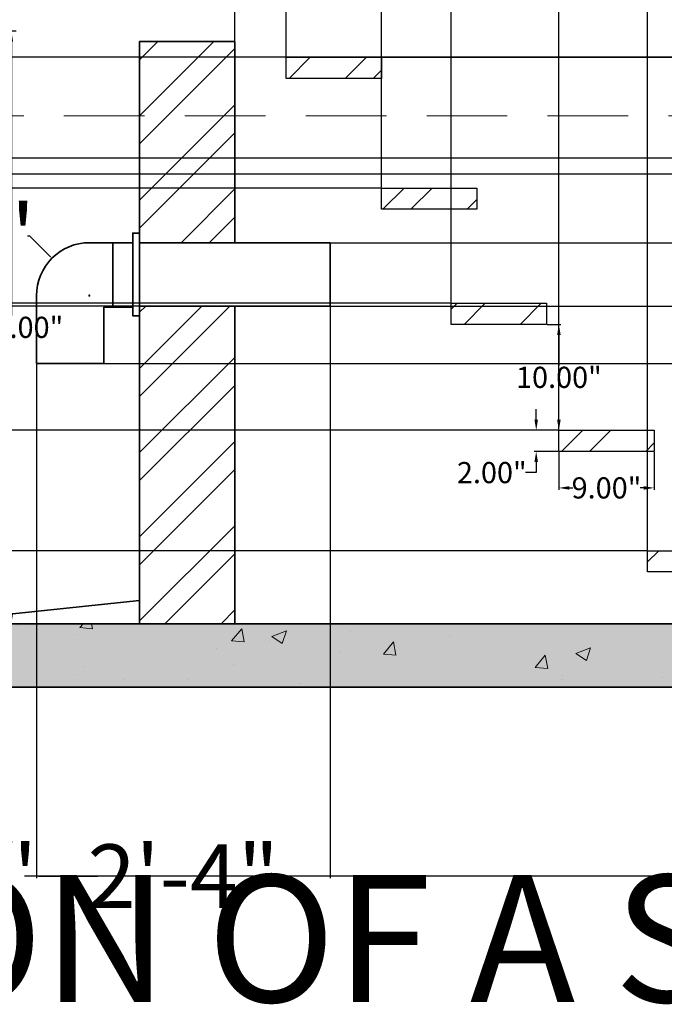
# Model space of a CAD drawing. Units: inches. Extents: x -34 to 285, y -151 to 155.
# Tile 6 of 10: x 129 to 189, y -151 to -58. Entities that reach past the tile are written whole.
import ezdxf

# ---------------------------------------------------------------- set-up
doc = ezdxf.new("R2010")
doc.units = ezdxf.units.IN
doc.header["$MEASUREMENT"] = 0
doc.linetypes.add('DASHED', pattern=[19.05, 12.7, -6.35])
for name, color, linetype, lineweight in [('A-ANNO-DIMS', 2, 'Continuous', 18), ('A-ANNO-TEXT', 7, 'Continuous', 25), ('A-DETL', 7, 'Continuous', 35), ('A-DETL-HIDN', 8, 'DASHED', 18), ('A-DETL-PATT', 8, 'Continuous', 18), ('A-FLOR-STRS', 3, 'Continuous', 25), ('P-SANR-PIPE', 4, 'Continuous', 35)]:
    doc.layers.add(name, color=color, linetype=linetype, lineweight=lineweight)
doc.styles.get("Standard").update_dxf_attribs({"font": 'arial.ttf'})
doc.dimstyles.get("Standard").update_dxf_attribs({"dimtxt": 6, "dimasz": 0.18, "dimexe": 0.18, "dimexo": 0.0625, "dimgap": 0.09, "dimtad": 0, "dimtih": 1, "dimtoh": 1, "dimzin": 0, "dimdsep": 46, "dimlunit": 3, "dimtxsty": 'Standard', "dimcen": 0.09, "dimadec": 0, "dimazin": 0, "dimtfac": 1, "dimtofl": 0, "dimtmove": 0, "dimatfit": 3, "dimfxl": 1, "dimtolj": 1, "dimtzin": 0, "dimarcsym": 0})

# ---------------------------------------------------------------- blocks, each defined once
blk = doc.blocks.new('*D29')
at = {"layer": 'A-ANNO-DIMS', "color": 0, "lineweight": -2, "transparency": 16777216}
for p, q in [((128.176, -58.969), (127.544, -58.969)), ((127.724, -59.969), (127.724, -85.858)), ((127.724, -113.969), (127.724, -88.08)), ((128.176, -114.969), (127.544, -114.969))]:
    blk.add_line(p, q, dxfattribs=at)
at = {"layer": 'A-ANNO-DIMS', "color": 0, "transparency": 16777216}
for points in [[(127.557, -59.969), (127.891, -59.969), (127.724, -58.969)], [(127.557, -113.969), (127.891, -113.969), (127.724, -114.969)]]:
    blk.add_solid(points, dxfattribs=at)
at = {"layer": 'Defpoints', "color": 0, "transparency": 16777216}
for p in [(128.239, -58.969), (127.724, -114.969), (128.239, -114.969)]:
    blk.add_point(p, dxfattribs=at)
at = {"layer": 'A-ANNO-DIMS', "color": 0, "transparency": 16777216, "insert": (127.724, -86.969), "char_height": 2, "attachment_point": 5}
blk.add_mtext('\\A1;4\'-8.00"', dxfattribs=at)
blk = doc.blocks.new('*D32')
at = {"layer": 'A-ANNO-DIMS', "color": 0, "lineweight": -2, "transparency": 16777216}
for p, q in [((178.365, -86.693), (179.662, -86.693)), ((179.482, -87.693), (179.482, -90.582)), ((179.482, -95.693), (179.482, -92.804)), ((179.544, -96.693), (179.662, -96.693))]:
    blk.add_line(p, q, dxfattribs=at)
at = {"layer": 'A-ANNO-DIMS', "color": 0, "transparency": 16777216}
for points in [[(179.315, -87.693), (179.648, -87.693), (179.482, -86.693)], [(179.315, -95.693), (179.648, -95.693), (179.482, -96.693)]]:
    blk.add_solid(points, dxfattribs=at)
at = {"layer": 'Defpoints', "color": 0, "transparency": 16777216}
for p in [(178.303, -86.693), (179.482, -96.693), (179.482, -96.693)]:
    blk.add_point(p, dxfattribs=at)
at = {"layer": 'A-ANNO-DIMS', "color": 0, "transparency": 16777216, "insert": (179.482, -91.693), "char_height": 2, "attachment_point": 5}
blk.add_mtext('\\A1;10.00"', dxfattribs=at)
blk = doc.blocks.new('*D33')
at = {"layer": 'A-ANNO-DIMS', "color": 0, "lineweight": -2, "transparency": 16777216}
for p, q in [((179.482, -98.755), (179.482, -102.319)), ((188.482, -98.755), (188.482, -102.319)), ((180.482, -102.139), (180.8, -102.139)), ((187.482, -102.139), (187.163, -102.139))]:
    blk.add_line(p, q, dxfattribs=at)
at = {"layer": 'A-ANNO-DIMS', "color": 0, "transparency": 16777216}
for points in [[(180.482, -101.973), (180.482, -102.306), (179.482, -102.139)], [(187.482, -101.973), (187.482, -102.306), (188.482, -102.139)]]:
    blk.add_solid(points, dxfattribs=at)
at = {"layer": 'Defpoints', "color": 0, "transparency": 16777216}
for p in [(179.482, -98.693), (188.482, -98.693), (188.482, -102.139)]:
    blk.add_point(p, dxfattribs=at)
at = {"layer": 'A-ANNO-DIMS', "color": 0, "transparency": 16777216, "insert": (183.982, -102.139), "char_height": 2, "attachment_point": 5}
blk.add_mtext('\\A1;9.00"', dxfattribs=at)
blk = doc.blocks.new('*D34')
at = {"layer": 'A-ANNO-DIMS', "color": 0, "lineweight": -2, "transparency": 16777216}
for p, q in [((177.338, -95.693), (177.338, -94.693)), ((179.419, -96.693), (177.158, -96.693)), ((179.419, -98.693), (177.158, -98.693)), ((177.338, -99.693), (177.338, -100.693)), ((177.338, -100.693), (176.338, -100.693))]:
    blk.add_line(p, q, dxfattribs=at)
at = {"layer": 'A-ANNO-DIMS', "color": 0, "transparency": 16777216}
for points in [[(177.171, -95.693), (177.504, -95.693), (177.338, -96.693)], [(177.171, -99.693), (177.504, -99.693), (177.338, -98.693)]]:
    blk.add_solid(points, dxfattribs=at)
at = {"layer": 'Defpoints', "color": 0, "transparency": 16777216}
for p in [(179.482, -96.693), (177.338, -98.693), (179.482, -98.693)]:
    blk.add_point(p, dxfattribs=at)
at = {"layer": 'A-ANNO-DIMS', "color": 0, "transparency": 16777216, "insert": (173.139, -100.693), "char_height": 2, "attachment_point": 5}
blk.add_mtext('\\A1;2.00"', dxfattribs=at)
blk = doc.blocks.new('*D48')
at = {"layer": 'A-ANNO-DIMS', "color": 0, "lineweight": -2, "transparency": 16777216}
for p, q in [((22.846, -121.031), (22.846, -138.999)), ((214.846, -121.031), (214.846, -138.999)), ((23.026, -138.819), (108.733, -138.819)), ((214.666, -138.819), (128.959, -138.819))]:
    blk.add_line(p, q, dxfattribs=at)
at = {"layer": 'A-ANNO-DIMS', "color": 0, "transparency": 16777216}
for points in [[(23.026, -138.789), (23.026, -138.849), (22.846, -138.819)], [(214.666, -138.789), (214.666, -138.849), (214.846, -138.819)]]:
    blk.add_solid(points, dxfattribs=at)
at = {"layer": 'Defpoints', "color": 0, "transparency": 16777216}
for p in [(22.846, -120.969), (214.846, -120.969), (214.846, -138.819)]:
    blk.add_point(p, dxfattribs=at)
at = {"layer": 'A-ANNO-DIMS', "color": 0, "transparency": 16777216, "insert": (118.846, -138.819), "char_height": 6, "attachment_point": 5}
blk.add_mtext('\\A1;16\'-0"', dxfattribs=at)
blk = doc.blocks.new('*D59')
at = {"layer": 'A-ANNO-DIMS', "color": 0, "lineweight": -2, "transparency": 16777216}
for p, q in [((83.148, -48.969), (241.637, -48.969)), ((241.457, -49.149), (241.457, -52)), ((241.457, -61.235), (241.457, -58.384)), ((89.009, -61.415), (241.637, -61.415))]:
    blk.add_line(p, q, dxfattribs=at)
at = {"layer": 'A-ANNO-DIMS', "color": 0, "transparency": 16777216}
for points in [[(241.427, -49.149), (241.487, -49.149), (241.457, -48.969)], [(241.427, -61.235), (241.487, -61.235), (241.457, -61.415)]]:
    blk.add_solid(points, dxfattribs=at)
at = {"layer": 'Defpoints', "color": 0, "transparency": 16777216}
for p in [(83.086, -48.969), (88.947, -61.415), (241.457, -61.415)]:
    blk.add_point(p, dxfattribs=at)
at = {"layer": 'A-ANNO-DIMS', "color": 0, "transparency": 16777216, "insert": (241.457, -55.192), "char_height": 6, "attachment_point": 5}
blk.add_mtext('\\A1;1\'-0 1/2"', dxfattribs=at)
blk = doc.blocks.new('*D61')
at = {"layer": 'A-ANNO-DIMS', "color": 0, "lineweight": -2, "transparency": 16777216}
for p, q in [((148.846, -59.906), (148.846, -18.978)), ((149.026, -19.158), (153.535, -19.158)), ((153.715, -61.389), (153.715, -18.978)), ((153.715, -19.158), (153.895, -19.158))]:
    blk.add_line(p, q, dxfattribs=at)
at = {"layer": 'A-ANNO-DIMS', "color": 0, "transparency": 16777216}
for points in [[(149.026, -19.128), (149.026, -19.188), (148.846, -19.158)], [(153.535, -19.128), (153.535, -19.188), (153.715, -19.158)]]:
    blk.add_solid(points, dxfattribs=at)
at = {"layer": 'Defpoints', "color": 0, "transparency": 16777216}
for p in [(153.715, -19.158), (148.846, -59.969), (153.715, -61.451)]:
    blk.add_point(p, dxfattribs=at)
at = {"layer": 'A-ANNO-DIMS', "color": 0, "transparency": 16777216, "insert": (161.96, -19.158), "char_height": 6, "attachment_point": 5}
blk.add_mtext('\\A1;0\'-5"', dxfattribs=at)
blk = doc.blocks.new('*D62')
at = {"layer": 'A-ANNO-DIMS', "color": 0, "lineweight": -2, "transparency": 16777216}
for p, q in [((155.218, -48.969), (241.637, -48.969)), ((241.457, -49.149), (241.457, -52.018)), ((241.457, -61.271), (241.457, -58.402)), ((153.777, -61.451), (241.637, -61.451))]:
    blk.add_line(p, q, dxfattribs=at)
at = {"layer": 'A-ANNO-DIMS', "color": 0, "transparency": 16777216}
for points in [[(241.427, -49.149), (241.487, -49.149), (241.457, -48.969)], [(241.427, -61.271), (241.487, -61.271), (241.457, -61.451)]]:
    blk.add_solid(points, dxfattribs=at)
at = {"layer": 'Defpoints', "color": 0, "transparency": 16777216}
for p in [(155.156, -48.969), (153.715, -61.451), (241.457, -61.451)]:
    blk.add_point(p, dxfattribs=at)
at = {"layer": 'A-ANNO-DIMS', "color": 0, "transparency": 16777216, "insert": (241.457, -55.21), "char_height": 6, "attachment_point": 5}
blk.add_mtext('\\A1;1\'-0 1/2"', dxfattribs=at)
blk = doc.blocks.new('*D63')
at = {"layer": 'A-ANNO-DIMS', "color": 0, "lineweight": -2, "transparency": 16777216}
for p, q in [((157.846, -79.031), (157.846, -138.999)), ((130.096, -90.432), (130.096, -138.999)), ((130.276, -138.819), (135.855, -138.819)), ((157.666, -138.819), (152.087, -138.819))]:
    blk.add_line(p, q, dxfattribs=at)
at = {"layer": 'A-ANNO-DIMS', "color": 0, "transparency": 16777216}
for points in [[(130.276, -138.789), (130.276, -138.849), (130.096, -138.819)], [(157.666, -138.789), (157.666, -138.849), (157.846, -138.819)]]:
    blk.add_solid(points, dxfattribs=at)
at = {"layer": 'Defpoints', "color": 0, "transparency": 16777216}
for p in [(157.846, -78.969), (130.096, -90.369), (157.846, -138.819)]:
    blk.add_point(p, dxfattribs=at)
at = {"layer": 'A-ANNO-DIMS', "color": 0, "transparency": 16777216, "insert": (143.971, -138.819), "char_height": 6, "attachment_point": 5}
blk.add_mtext('\\A1;2\'-4"', dxfattribs=at)
blk = doc.blocks.new('*D64')
at = {"layer": 'A-ANNO-DIMS', "color": 0, "lineweight": -2, "transparency": 16777216}
for p, q in [((157.783, -84.969), (0.722, -84.969)), ((0.902, -85.149), (0.902, -96.816)), ((0.902, -114.789), (0.902, -103.122)), ((148.783, -114.969), (0.722, -114.969))]:
    blk.add_line(p, q, dxfattribs=at)
at = {"layer": 'A-ANNO-DIMS', "color": 0, "transparency": 16777216}
for points in [[(0.872, -85.149), (0.932, -85.149), (0.902, -84.969)], [(0.872, -114.789), (0.932, -114.789), (0.902, -114.969)]]:
    blk.add_solid(points, dxfattribs=at)
at = {"layer": 'Defpoints', "color": 0, "transparency": 16777216}
for p in [(157.846, -84.969), (0.902, -114.969), (148.846, -114.969)]:
    blk.add_point(p, dxfattribs=at)
at = {"layer": 'A-ANNO-DIMS', "color": 0, "transparency": 16777216, "insert": (0.902, -99.969), "char_height": 6, "attachment_point": 5}
blk.add_mtext('\\A1;2\'-6"', dxfattribs=at)
blk = doc.blocks.new('*D65')
at = {"layer": 'A-ANNO-DIMS', "color": 0, "lineweight": -2, "transparency": 16777216}
for p, q in [((130.158, -90.369), (241.637, -90.369)), ((241.457, -90.549), (241.457, -99.477)), ((241.457, -114.789), (241.457, -105.861)), ((139.908, -114.969), (241.637, -114.969))]:
    blk.add_line(p, q, dxfattribs=at)
at = {"layer": 'A-ANNO-DIMS', "color": 0, "transparency": 16777216}
for points in [[(241.427, -90.549), (241.487, -90.549), (241.457, -90.369)], [(241.427, -114.789), (241.487, -114.789), (241.457, -114.969)]]:
    blk.add_solid(points, dxfattribs=at)
at = {"layer": 'Defpoints', "color": 0, "transparency": 16777216}
for p in [(130.096, -90.369), (139.846, -114.969), (241.457, -114.969)]:
    blk.add_point(p, dxfattribs=at)
at = {"layer": 'A-ANNO-DIMS', "color": 0, "transparency": 16777216, "insert": (241.457, -102.669), "char_height": 6, "attachment_point": 5}
blk.add_mtext('\\A1;2\'-0 1/2"', dxfattribs=at)
blk = doc.blocks.new('*D66')
at = {"layer": 'A-ANNO-DIMS', "color": 0, "lineweight": -2, "transparency": 16777216}
for p, q in [((157.908, -78.969), (241.637, -78.969)), ((241.457, -79.149), (241.457, -84.789)), ((157.908, -84.969), (241.637, -84.969)), ((241.457, -85.149), (241.277, -85.149)), ((241.457, -84.969), (241.457, -85.149))]:
    blk.add_line(p, q, dxfattribs=at)
at = {"layer": 'A-ANNO-DIMS', "color": 0, "transparency": 16777216}
for points in [[(241.427, -79.149), (241.487, -79.149), (241.457, -78.969)], [(241.427, -84.789), (241.487, -84.789), (241.457, -84.969)]]:
    blk.add_solid(points, dxfattribs=at)
at = {"layer": 'Defpoints', "color": 0, "transparency": 16777216}
for p in [(157.846, -78.969), (157.846, -84.969), (241.457, -84.969)]:
    blk.add_point(p, dxfattribs=at)
at = {"layer": 'A-ANNO-DIMS', "color": 0, "transparency": 16777216, "insert": (233.213, -85.149), "char_height": 6, "attachment_point": 5}
blk.add_mtext('\\A1;0\'-6"', dxfattribs=at)
blk = doc.blocks.new('*D69')
at = {"layer": 'A-ANNO-DIMS', "color": 0, "lineweight": -2, "transparency": 16777216}
for p, q in [((97.668, -81.282), (97.668, -18.978)), ((97.848, -19.158), (105.119, -19.158)), ((105.299, -90.467), (105.299, -18.978)), ((105.299, -19.158), (105.479, -19.158))]:
    blk.add_line(p, q, dxfattribs=at)
at = {"layer": 'A-ANNO-DIMS', "color": 0, "transparency": 16777216}
for points in [[(97.848, -19.128), (97.848, -19.188), (97.668, -19.158)], [(105.119, -19.128), (105.119, -19.188), (105.299, -19.158)]]:
    blk.add_solid(points, dxfattribs=at)
at = {"layer": 'Defpoints', "color": 0, "transparency": 16777216}
for p in [(105.299, -19.158), (97.668, -81.345), (105.299, -90.53)]:
    blk.add_point(p, dxfattribs=at)
at = {"layer": 'A-ANNO-DIMS', "color": 0, "transparency": 16777216, "insert": (120.534, -19.158), "char_height": 6, "attachment_point": 5}
blk.add_mtext('\\A1;0\'-7 1/2"', dxfattribs=at)
blk = doc.blocks.new('*D70')
at = {"layer": 'A-ANNO-DIMS', "color": 0, "lineweight": -2, "transparency": 16777216}
for p, q in [((105.299, -90.467), (105.299, -18.978)), ((105.479, -19.158), (115.871, -19.158)), ((116.051, -97.053), (116.051, -18.978)), ((116.051, -19.158), (116.231, -19.158))]:
    blk.add_line(p, q, dxfattribs=at)
at = {"layer": 'A-ANNO-DIMS', "color": 0, "transparency": 16777216}
for points in [[(105.479, -19.128), (105.479, -19.188), (105.299, -19.158)], [(115.871, -19.128), (115.871, -19.188), (116.051, -19.158)]]:
    blk.add_solid(points, dxfattribs=at)
at = {"layer": 'Defpoints', "color": 0, "transparency": 16777216}
for p in [(116.051, -19.158), (105.299, -90.53), (116.051, -97.116)]:
    blk.add_point(p, dxfattribs=at)
at = {"layer": 'A-ANNO-DIMS', "color": 0, "transparency": 16777216, "insert": (126.627, -19.158), "char_height": 6, "attachment_point": 5}
blk.add_mtext('\\A1;0\'-11"', dxfattribs=at)
blk = doc.blocks.new('*D71')
at = {"layer": 'A-ANNO-DIMS', "color": 0, "lineweight": -2, "transparency": 16777216}
for p, q in [((116.051, -97.053), (116.051, -18.978)), ((116.231, -19.158), (121.719, -19.158)), ((121.899, -103.966), (121.899, -18.978)), ((121.899, -19.158), (122.079, -19.158))]:
    blk.add_line(p, q, dxfattribs=at)
at = {"layer": 'A-ANNO-DIMS', "color": 0, "transparency": 16777216}
for points in [[(116.231, -19.128), (116.231, -19.188), (116.051, -19.158)], [(121.719, -19.128), (121.719, -19.188), (121.899, -19.158)]]:
    blk.add_solid(points, dxfattribs=at)
at = {"layer": 'Defpoints', "color": 0, "transparency": 16777216}
for p in [(121.899, -19.158), (116.051, -97.116), (121.899, -104.028)]:
    blk.add_point(p, dxfattribs=at)
at = {"layer": 'A-ANNO-DIMS', "color": 0, "transparency": 16777216, "insert": (130.144, -19.158), "char_height": 6, "attachment_point": 5}
blk.add_mtext('\\A1;0\'-6"', dxfattribs=at)
blk = doc.blocks.new('*D78')
at = {"layer": 'A-ANNO-DIMS', "color": 0, "lineweight": -2, "transparency": 16777216}
for p, q in [((96.293, -70.947), (241.637, -70.947)), ((241.457, -71.127), (241.457, -72.29)), ((96.293, -72.47), (241.637, -72.47)), ((241.457, -72.47), (241.457, -72.65)), ((241.457, -72.65), (241.277, -72.65))]:
    blk.add_line(p, q, dxfattribs=at)
at = {"layer": 'A-ANNO-DIMS', "color": 0, "transparency": 16777216}
for points in [[(241.427, -71.127), (241.487, -71.127), (241.457, -70.947)], [(241.427, -72.29), (241.487, -72.29), (241.457, -72.47)]]:
    blk.add_solid(points, dxfattribs=at)
at = {"layer": 'Defpoints', "color": 0, "transparency": 16777216}
for p in [(96.231, -70.947), (96.231, -72.47), (241.457, -72.47)]:
    blk.add_point(p, dxfattribs=at)
at = {"layer": 'A-ANNO-DIMS', "color": 0, "transparency": 16777216, "insert": (226.222, -72.65), "char_height": 6, "attachment_point": 5}
blk.add_mtext('\\A1;0\'-1 1/2"', dxfattribs=at)
blk = doc.blocks.new('*D79')
at = {"layer": 'A-ANNO-DIMS', "color": 0, "lineweight": -2, "transparency": 16777216}
for p, q in [((153.715, -61.389), (153.715, -18.978)), ((153.895, -19.158), (162.535, -19.158)), ((162.715, -73.74), (162.715, -18.978)), ((162.715, -19.158), (162.895, -19.158))]:
    blk.add_line(p, q, dxfattribs=at)
at = {"layer": 'A-ANNO-DIMS', "color": 0, "transparency": 16777216}
for points in [[(153.895, -19.128), (153.895, -19.188), (153.715, -19.158)], [(162.535, -19.128), (162.535, -19.188), (162.715, -19.158)]]:
    blk.add_solid(points, dxfattribs=at)
at = {"layer": 'Defpoints', "color": 0, "transparency": 16777216}
for p in [(162.715, -19.158), (153.715, -61.451), (162.715, -73.803)]:
    blk.add_point(p, dxfattribs=at)
at = {"layer": 'A-ANNO-DIMS', "color": 0, "transparency": 16777216, "insert": (170.96, -19.158), "char_height": 6, "attachment_point": 5}
blk.add_mtext('\\A1;0\'-9"', dxfattribs=at)
blk = doc.blocks.new('*D80')
at = {"layer": 'A-ANNO-DIMS', "color": 0, "lineweight": -2, "transparency": 16777216}
for p, q in [((162.715, -73.74), (162.715, -18.978)), ((162.895, -19.158), (169.123, -19.158)), ((169.303, -84.63), (169.303, -18.978)), ((169.303, -19.158), (169.483, -19.158))]:
    blk.add_line(p, q, dxfattribs=at)
at = {"layer": 'A-ANNO-DIMS', "color": 0, "transparency": 16777216}
for points in [[(162.895, -19.128), (162.895, -19.188), (162.715, -19.158)], [(169.123, -19.128), (169.123, -19.188), (169.303, -19.158)]]:
    blk.add_solid(points, dxfattribs=at)
at = {"layer": 'Defpoints', "color": 0, "transparency": 16777216}
for p in [(169.303, -19.158), (162.715, -73.803), (169.303, -84.693)]:
    blk.add_point(p, dxfattribs=at)
at = {"layer": 'A-ANNO-DIMS', "color": 0, "transparency": 16777216, "insert": (184.538, -19.158), "char_height": 6, "attachment_point": 5}
blk.add_mtext('\\A1;0\'-6 1/2"', dxfattribs=at)
blk = doc.blocks.new('*D81')
at = {"layer": 'A-ANNO-DIMS', "color": 0, "lineweight": -2, "transparency": 16777216}
for p, q in [((169.303, -84.63), (169.303, -18.978)), ((169.483, -19.158), (179.302, -19.158)), ((179.482, -96.63), (179.482, -18.978)), ((179.482, -19.158), (179.662, -19.158))]:
    blk.add_line(p, q, dxfattribs=at)
at = {"layer": 'A-ANNO-DIMS', "color": 0, "transparency": 16777216}
for points in [[(169.483, -19.128), (169.483, -19.188), (169.303, -19.158)], [(179.302, -19.128), (179.302, -19.188), (179.482, -19.158)]]:
    blk.add_solid(points, dxfattribs=at)
at = {"layer": 'Defpoints', "color": 0, "transparency": 16777216}
for p in [(179.482, -19.158), (169.303, -84.693), (179.482, -96.693)]:
    blk.add_point(p, dxfattribs=at)
at = {"layer": 'A-ANNO-DIMS', "color": 0, "transparency": 16777216, "insert": (190.057, -19.158), "char_height": 6, "attachment_point": 5}
blk.add_mtext('\\A1;0\'-10"', dxfattribs=at)
blk = doc.blocks.new('*D82')
at = {"layer": 'A-ANNO-DIMS', "color": 0, "lineweight": -2, "transparency": 16777216}
for p, q in [((179.482, -96.63), (179.482, -18.978)), ((179.662, -19.158), (187.666, -19.158)), ((187.846, -108.007), (187.846, -18.978)), ((187.846, -19.158), (188.026, -19.158))]:
    blk.add_line(p, q, dxfattribs=at)
at = {"layer": 'A-ANNO-DIMS', "color": 0, "transparency": 16777216}
for points in [[(179.662, -19.128), (179.662, -19.188), (179.482, -19.158)], [(187.666, -19.128), (187.666, -19.188), (187.846, -19.158)]]:
    blk.add_solid(points, dxfattribs=at)
at = {"layer": 'Defpoints', "color": 0, "transparency": 16777216}
for p in [(187.846, -19.158), (179.482, -96.693), (187.846, -108.07)]:
    blk.add_point(p, dxfattribs=at)
at = {"layer": 'A-ANNO-DIMS', "color": 0, "transparency": 16777216, "insert": (203.081, -19.158), "char_height": 6, "attachment_point": 5}
blk.add_mtext('\\A1;0\'-8 1/2"', dxfattribs=at)
blk = doc.blocks.new('*D83')
at = {"layer": 'A-ANNO-DIMS', "color": 0, "lineweight": -2, "transparency": 16777216}
for p, q in [((153.652, -61.451), (0.722, -61.451)), ((0.902, -61.631), (0.902, -64.435)), ((0.902, -73.623), (0.902, -70.819)), ((162.652, -73.803), (0.722, -73.803))]:
    blk.add_line(p, q, dxfattribs=at)
at = {"layer": 'A-ANNO-DIMS', "color": 0, "transparency": 16777216}
for points in [[(0.872, -61.631), (0.932, -61.631), (0.902, -61.451)], [(0.872, -73.623), (0.932, -73.623), (0.902, -73.803)]]:
    blk.add_solid(points, dxfattribs=at)
at = {"layer": 'Defpoints', "color": 0, "transparency": 16777216}
for p in [(153.715, -61.451), (0.902, -73.803), (162.715, -73.803)]:
    blk.add_point(p, dxfattribs=at)
at = {"layer": 'A-ANNO-DIMS', "color": 0, "transparency": 16777216, "insert": (0.902, -67.627), "char_height": 6, "attachment_point": 5}
blk.add_mtext('\\A1;1\'-0 1/2"', dxfattribs=at)
blk = doc.blocks.new('*D84')
at = {"layer": 'A-ANNO-DIMS', "color": 0, "lineweight": -2, "transparency": 16777216}
for p, q in [((162.652, -73.803), (0.722, -73.803)), ((0.902, -73.983), (0.902, -76.094)), ((0.902, -84.513), (0.902, -82.401)), ((169.24, -84.693), (0.722, -84.693))]:
    blk.add_line(p, q, dxfattribs=at)
at = {"layer": 'A-ANNO-DIMS', "color": 0, "transparency": 16777216}
for points in [[(0.872, -73.983), (0.932, -73.983), (0.902, -73.803)], [(0.872, -84.513), (0.932, -84.513), (0.902, -84.693)]]:
    blk.add_solid(points, dxfattribs=at)
at = {"layer": 'Defpoints', "color": 0, "transparency": 16777216}
for p in [(162.715, -73.803), (0.902, -84.693), (169.303, -84.693)]:
    blk.add_point(p, dxfattribs=at)
at = {"layer": 'A-ANNO-DIMS', "color": 0, "transparency": 16777216, "insert": (0.902, -79.248), "char_height": 6, "attachment_point": 5}
blk.add_mtext('\\A1;0\'-11"', dxfattribs=at)
blk = doc.blocks.new('*D85')
at = {"layer": 'A-ANNO-DIMS', "color": 0, "lineweight": -2, "transparency": 16777216}
for p, q in [((169.24, -84.693), (0.722, -84.693)), ((0.902, -84.873), (0.902, -87.539)), ((0.902, -96.513), (0.902, -93.846)), ((179.419, -96.693), (0.722, -96.693))]:
    blk.add_line(p, q, dxfattribs=at)
at = {"layer": 'A-ANNO-DIMS', "color": 0, "transparency": 16777216}
for points in [[(0.872, -84.873), (0.932, -84.873), (0.902, -84.693)], [(0.872, -96.513), (0.932, -96.513), (0.902, -96.693)]]:
    blk.add_solid(points, dxfattribs=at)
at = {"layer": 'Defpoints', "color": 0, "transparency": 16777216}
for p in [(169.303, -84.693), (0.902, -96.693), (179.482, -96.693)]:
    blk.add_point(p, dxfattribs=at)
at = {"layer": 'A-ANNO-DIMS', "color": 0, "transparency": 16777216, "insert": (0.902, -90.693), "char_height": 6, "attachment_point": 5}
blk.add_mtext('\\A1;1\'-0"', dxfattribs=at)
blk = doc.blocks.new('*D86')
at = {"layer": 'A-ANNO-DIMS', "color": 0, "lineweight": -2, "transparency": 16777216}
for p, q in [((179.419, -96.693), (0.722, -96.693)), ((0.902, -96.873), (0.902, -99.189)), ((0.902, -107.89), (0.902, -105.574)), ((187.783, -108.07), (0.722, -108.07))]:
    blk.add_line(p, q, dxfattribs=at)
at = {"layer": 'A-ANNO-DIMS', "color": 0, "transparency": 16777216}
for points in [[(0.872, -96.873), (0.932, -96.873), (0.902, -96.693)], [(0.872, -107.89), (0.932, -107.89), (0.902, -108.07)]]:
    blk.add_solid(points, dxfattribs=at)
at = {"layer": 'Defpoints', "color": 0, "transparency": 16777216}
for p in [(179.482, -96.693), (0.902, -108.07), (187.846, -108.07)]:
    blk.add_point(p, dxfattribs=at)
at = {"layer": 'A-ANNO-DIMS', "color": 0, "transparency": 16777216, "insert": (0.902, -102.381), "char_height": 6, "attachment_point": 5}
blk.add_mtext('\\A1;0\'-11 1/2"', dxfattribs=at)
blk = doc.blocks.new('*D87')
at = {"layer": 'A-ANNO-DIMS', "color": 0, "lineweight": -2, "transparency": 16777216}
for p, q in [((187.783, -108.07), (0.722, -108.07)), ((0.902, -108.25), (0.902, -108.366)), ((196.783, -114.969), (0.722, -114.969)), ((0.902, -114.789), (0.902, -114.673))]:
    blk.add_line(p, q, dxfattribs=at)
at = {"layer": 'A-ANNO-DIMS', "color": 0, "transparency": 16777216}
for points in [[(0.872, -108.25), (0.932, -108.25), (0.902, -108.07)], [(0.872, -114.789), (0.932, -114.789), (0.902, -114.969)]]:
    blk.add_solid(points, dxfattribs=at)
at = {"layer": 'Defpoints', "color": 0, "transparency": 16777216}
for p in [(187.846, -108.07), (0.902, -114.969), (196.846, -114.969)]:
    blk.add_point(p, dxfattribs=at)
at = {"layer": 'A-ANNO-DIMS', "color": 0, "transparency": 16777216, "insert": (0.902, -111.519), "char_height": 6, "attachment_point": 5}
blk.add_mtext('\\A1;0\'-7"', dxfattribs=at)
blk = doc.blocks.new('*D93')
at = {"layer": 'A-ANNO-DIMS', "color": 0, "lineweight": -2, "transparency": 16777216}
for p, q in [((129.261, -78.309), (129.441, -78.309)), ((129.441, -78.309), (131.435, -80.304)), ((135.006, -83.969), (135.186, -83.969)), ((135.096, -84.059), (135.096, -83.879))]:
    blk.add_line(p, q, dxfattribs=at)
at = {"layer": 'A-ANNO-DIMS', "color": 0, "transparency": 16777216}
blk.add_solid([(131.456, -80.283), (131.413, -80.326), (131.562, -80.432)], dxfattribs=at)
at = {"layer": 'Defpoints', "color": 0, "transparency": 16777216}
for p in [(131.562, -80.432), (135.096, -83.969)]:
    blk.add_point(p, dxfattribs=at)
at = {"layer": 'A-ANNO-DIMS', "color": 0, "transparency": 16777216, "insert": (118.326, -78.309), "char_height": 6, "attachment_point": 5}
blk.add_mtext('\\A1;R0\'-5"', dxfattribs=at)

msp = doc.modelspace()

# ---------------------------------------------------------------- hatches: boundary and pattern name
at = {"layer": 'A-DETL-PATT'}
h = msp.add_hatch(dxfattribs=at)
h.set_pattern_fill('AR-CONC', color=256, scale=0.4)
h.set_pattern_definition([(50, (0, 0), (2.86904, -0.251009), [0.3, -3.3]), (355, (0, 0), (-0.555005, 3.00877), [0.24, -2.64]), (100.4514, (0.239, -0.021), (2.314035, 2.75776), [0.25496, -2.80457]), (46.1842, (0, 0.8), (4.268965, -0.662077), [0.45, -4.95]), (96.6356, (0.3557, 0.745), (3.73865, 3.896474), [0.38244, -4.206855]), (351.1842, (0, 0.8), (3.73865, 3.896474), [0.36, -3.96]), (21, (0.4, 0.6), (2.387628, -1.610476), [0.3, -3.3]), (326, (0.4, 0.6), (0.97326, 2.9006), [0.24, -2.64]), (71.4514, (0.599, 0.4658), (3.36089, 1.290125), [0.25496, -2.80457]), (37.5, (0, 0), (0.0486394, 1.3315754), [0, -2.608, 0, -2.68, 0, -2.65]), (7.5, (0, 0), (1.052278, 1.577647), [0, -1.528, 0, -2.548, 0, -1.01]), (327.5, (-0.892, 0), (2.1352897, -0.0902195), [0, -1, 0, -3.12, 0, -4.14]), (317.5, (-1.292, 0), (2.332745, 0.40042), [0, -1.3, 0, -2.072, 0, -2.94])])
h.paths.add_polyline_path([(214.846, -48.969), (214.846, -42.969), (184.518, -42.969), (184.518, -48.969)])
h.paths.add_polyline_path([(122.241, -42.969), (122.241, -48.969), (155.156, -48.969), (155.156, -42.969)])
h.paths.add_polyline_path([(214.846, -114.969), (22.846, -114.969), (22.846, -120.969), (214.846, -120.969)])
h = msp.add_hatch(dxfattribs=at)
h.set_pattern_fill('ANSI32', color=256, scale=15)
h.paths.add_polyline_path([(148.846, -59.969), (139.846, -59.969), (139.846, -66.969), (148.846, -66.969)])
h.paths.add_polyline_path([(148.846, -66.969), (139.846, -66.969), (139.846, -78.969), (148.846, -78.969)])
h.paths.add_polyline_path([(148.846, -84.969), (139.846, -84.969), (139.846, -85.88), (139.846, -114.969), (148.846, -114.969)])
h.paths.add_polyline_path([(40.846, -65.853), (32.384, -65.853), (31.846, -65.853), (31.846, -114.969), (40.846, -114.969)])
h.paths.add_polyline_path([(40.846, -48.969), (31.846, -48.969), (31.846, -59.853), (40.846, -59.853)])
h = msp.add_hatch(dxfattribs=at)
h.set_pattern_fill('ANSI32', color=256, scale=15)
h.paths.add_polyline_path([(171.715, -73.803), (162.715, -73.803), (162.715, -75.803), (171.715, -75.803)])
h.paths.add_polyline_path([(178.303, -84.693), (169.303, -84.693), (169.303, -86.693), (178.303, -86.693)])
h.paths.add_polyline_path([(188.482, -96.693), (179.482, -96.693), (179.482, -98.693), (188.482, -98.693)])
h.paths.add_polyline_path([(196.846, -108.07), (187.846, -108.07), (187.846, -110.07), (196.846, -110.07)])
h.paths.add_polyline_path([(162.715, -61.451), (153.715, -61.451), (153.715, -63.451), (162.715, -63.451)])
h = msp.add_hatch(dxfattribs=at)
h.set_pattern_fill('AR-CONC', color=256, scale=2)
h.paths.add_polyline_path([(22.846, -114.969), (22.846, -120.969), (214.846, -120.969), (214.846, -114.969)])

# ---------------------------------------------------------------- linework, layer by layer
at = {"layer": 'A-DETL'}
for p, q in [((139.846, -59.969), (139.846, -114.969)), ((139.846, -59.969), (148.846, -59.969)), ((148.846, -59.969), (148.846, -78.969)), ((148.846, -84.969), (148.846, -114.969)), ((118.846, -114.969), (139.846, -112.768)), ((22.846, -114.969), (214.846, -114.969)), ((22.846, -120.969), (214.846, -120.969))]:
    msp.add_line(p, q, dxfattribs=at)
at = {"layer": 'A-DETL-HIDN', "ltscale": 0.6}
msp.add_line((75.547, -66.969), (214.207, -66.969), dxfattribs=at)
at = {"layer": 'A-FLOR-STRS'}
for points in [[(162.715, -63.451), (153.715, -63.451), (153.715, -61.451), (162.715, -61.451)], [(171.715, -75.803), (162.715, -75.803), (162.715, -73.803), (171.715, -73.803)], [(178.303, -86.693), (169.303, -86.693), (169.303, -84.693), (178.303, -84.693)], [(188.482, -98.693), (179.482, -98.693), (179.482, -96.693), (188.482, -96.693)], [(196.846, -110.07), (187.846, -110.07), (187.846, -108.07), (196.846, -108.07)]]:
    msp.add_lwpolyline(points, close=True, dxfattribs=at)
at = {"layer": 'P-SANR-PIPE'}
for p, q in [((137.312, -78.969), (139.203, -78.969)), ((139.846, -78.969), (148.846, -78.969)), ((139.203, -85.07), (136.479, -85.07)), ((136.479, -85.07), (136.479, -90.369)), ((137.512, -85.07), (137.312, -85.07)), ((136.479, -90.369), (130.096, -90.369))]:
    msp.add_line(p, q, dxfattribs=at)
msp.add_lwpolyline([(139.846, -78.063), (139.203, -78.063), (139.203, -85.88), (139.846, -85.88)], close=True, dxfattribs=at)
msp.add_lwpolyline([(139.203, -78.969), (135.096, -78.969, 0.414214), (130.096, -83.969), (130.096, -90.369)], format="xyb", dxfattribs=at)
for points in [[(137.312, -78.969), (137.312, -85.07)], [(148.846, -78.969), (157.846, -78.969), (157.846, -84.969), (139.846, -84.969)], [(148.846, -78.969), (157.846, -78.969), (157.846, -84.969), (148.846, -84.969)], [(148.846, -78.969), (157.846, -78.969), (157.846, -84.969), (148.846, -84.969)]]:
    msp.add_lwpolyline(points, dxfattribs=at)

# ---------------------------------------------------------------- texts
at = {"layer": 'A-ANNO-TEXT', "insert": (-34.52, -138.72), "char_height": 12, "attachment_point": 1}
msp.add_mtext_dynamic_manual_height_columns('SECTIONAL ELEVATION OF A SEPTIC TANK ', width=509.35271, gutter_width=1, heights=[0], dxfattribs=at)

# ---------------------------------------------------------------- dimensions: what is measured, and where the dimension line sits
at = {"layer": 'A-ANNO-DIMS'}
for base, p1, p2, override, picture, middle in [((105.299, -19.158), (97.668, -81.345), (105.299, -90.53), {"dimdec": 1, "dimlfac": 1, "dimrnd": 0, "dimzin": 1, "dimdsep": 46, "dimlunit": 4, "dimfrac": 2}, '*D69', (120.534, -19.158)), ((169.303, -19.158), (162.715, -73.803), (169.303, -84.693), {"dimdec": 1, "dimlfac": 1, "dimrnd": 0, "dimzin": 1, "dimdsep": 46, "dimlunit": 4, "dimfrac": 2}, '*D80', (184.538, -19.158)), ((187.846, -19.158), (179.482, -96.693), (187.846, -108.07), {"dimdec": 1, "dimlfac": 1, "dimrnd": 0, "dimzin": 1, "dimdsep": 46, "dimlunit": 4, "dimfrac": 2}, '*D82', (203.081, -19.158)), ((116.051, -19.158), (105.299, -90.53), (116.051, -97.116), {"dimdec": 1, "dimlfac": 1, "dimrnd": 0, "dimzin": 1, "dimdsep": 46, "dimlunit": 4, "dimfrac": 2}, '*D70', (126.627, -19.158)), ((121.899, -19.158), (116.051, -97.116), (121.899, -104.028), {"dimdec": 1, "dimlfac": 1, "dimrnd": 0, "dimzin": 1, "dimdsep": 46, "dimlunit": 4, "dimfrac": 2}, '*D71', (130.144, -19.158)), ((153.715, -19.158), (148.846, -59.969), (153.715, -61.451), {"dimdec": 1, "dimlfac": 1, "dimrnd": 0, "dimzin": 1, "dimdsep": 46, "dimlunit": 4, "dimfrac": 2}, '*D61', (161.96, -19.158)), ((162.715, -19.158), (153.715, -61.451), (162.715, -73.803), {"dimdec": 1, "dimlfac": 1, "dimrnd": 0, "dimzin": 1, "dimdsep": 46, "dimlunit": 4, "dimfrac": 2}, '*D79', (170.96, -19.158)), ((179.482, -19.158), (169.303, -84.693), (179.482, -96.693), {"dimdec": 1, "dimlfac": 1, "dimrnd": 0, "dimzin": 1, "dimdsep": 46, "dimlunit": 4, "dimfrac": 2}, '*D81', (190.057, -19.158)), ((157.8458, -138.819), (130.0957, -90.3694), (157.8458, -78.969), {"dimdec": 1, "dimlfac": 1, "dimrnd": 0, "dimzin": 1, "dimdsep": 46, "dimlunit": 4, "dimfrac": 2}, '*D63', (143.9707, -138.819)), ((188.482, -102.139), (179.482, -98.693), (188.482, -98.693), {"dimtxt": 2, "dimasz": 1, "dimclrd": 0, "dimclre": 0, "dimclrt": 0}, '*D33', (183.982, -102.139)), ((214.846, -138.819), (22.846, -120.969), (214.846, -120.969), {"dimdec": 1, "dimlfac": 1, "dimrnd": 0, "dimzin": 1, "dimdsep": 46, "dimlunit": 4, "dimfrac": 2}, '*D48', (118.846, -138.819))]:
    dim = msp.add_linear_dim(base=base, p1=p1, p2=p2, dimstyle='Standard', override=override, dxfattribs=at)
    dim.commit()
    dim.dimension.update_dxf_attribs({"geometry": picture, "text_midpoint": middle})
for base, p1, p2, override, picture, middle in [((241.457, -61.415), (83.086, -48.969), (88.947, -61.415), {"dimdec": 1, "dimlfac": 1, "dimrnd": 0, "dimzin": 1, "dimdsep": 46, "dimlunit": 4, "dimfrac": 2}, '*D59', (241.457, -55.192)), ((241.457, -61.451), (155.156, -48.969), (153.715, -61.451), {"dimdec": 1, "dimlfac": 1, "dimrnd": 0, "dimzin": 1, "dimdsep": 46, "dimlunit": 4, "dimfrac": 2}, '*D62', (241.457, -55.21)), ((0.902, -73.803), (153.715, -61.451), (162.715, -73.803), {"dimdec": 1, "dimlfac": 1, "dimrnd": 0, "dimzin": 1, "dimdsep": 46, "dimlunit": 4, "dimfrac": 2}, '*D83', (0.902, -67.627)), ((127.724, -114.969), (128.239, -58.969), (128.239, -114.969), {"dimtxt": 2, "dimasz": 1, "dimclrd": 0, "dimclre": 0, "dimclrt": 0}, '*D29', (127.724, -86.969)), ((241.457, -72.47), (96.231, -70.947), (96.231, -72.47), {"dimdec": 1, "dimlfac": 1, "dimrnd": 0, "dimzin": 1, "dimdsep": 46, "dimlunit": 4, "dimfrac": 2}, '*D78', (226.222, -72.65)), ((0.902, -84.693), (162.715, -73.803), (169.303, -84.693), {"dimdec": 1, "dimlfac": 1, "dimrnd": 0, "dimzin": 1, "dimdsep": 46, "dimlunit": 4, "dimfrac": 2}, '*D84', (0.902, -79.248)), ((241.457, -84.969), (157.846, -78.969), (157.846, -84.969), {"dimdec": 1, "dimlfac": 1, "dimrnd": 0, "dimzin": 1, "dimdsep": 46, "dimlunit": 4, "dimfrac": 2}, '*D66', (233.213, -85.149)), ((0.902, -96.693), (169.303, -84.693), (179.482, -96.693), {"dimdec": 1, "dimlfac": 1, "dimrnd": 0, "dimzin": 1, "dimdsep": 46, "dimlunit": 4, "dimfrac": 2}, '*D85', (0.902, -90.693)), ((0.902, -114.969), (157.846, -84.969), (148.846, -114.969), {"dimdec": 1, "dimlfac": 1, "dimrnd": 0, "dimzin": 1, "dimdsep": 46, "dimlunit": 4, "dimfrac": 2}, '*D64', (0.902, -99.969)), ((179.482, -96.693), (178.303, -86.693), (179.482, -96.693), {"dimtxt": 2, "dimasz": 1, "dimclrd": 0, "dimclre": 0, "dimclrt": 0}, '*D32', (179.482, -91.693)), ((241.457, -114.969), (130.096, -90.369), (139.846, -114.969), {"dimdec": 1, "dimlfac": 1, "dimrnd": 0, "dimzin": 1, "dimdsep": 46, "dimlunit": 4, "dimfrac": 2}, '*D65', (241.457, -102.669)), ((0.902, -108.07), (179.482, -96.693), (187.846, -108.07), {"dimdec": 1, "dimlfac": 1, "dimrnd": 0, "dimzin": 1, "dimdsep": 46, "dimlunit": 4, "dimfrac": 2}, '*D86', (0.902, -102.381)), ((177.338, -98.693), (179.482, -96.693), (179.482, -98.693), {"dimtxt": 2, "dimasz": 1, "dimclrd": 0, "dimclre": 0, "dimclrt": 0}, '*D34', (173.139, -100.693)), ((0.902, -114.969), (187.846, -108.07), (196.846, -114.969), {"dimdec": 1, "dimlfac": 1, "dimrnd": 0, "dimzin": 1, "dimdsep": 46, "dimlunit": 4, "dimfrac": 2}, '*D87', (0.902, -111.519))]:
    dim = msp.add_linear_dim(base=base, p1=p1, p2=p2, angle=90, dimstyle='Standard', override=override, dxfattribs=at)
    dim.commit()
    dim.dimension.update_dxf_attribs({"geometry": picture, "text_midpoint": middle})
dim = msp.add_radius_dim(center=(135.096, -83.969), mpoint=(131.562, -80.432), dimstyle='Standard', override={"dimdec": 1, "dimlfac": 1, "dimrnd": 0, "dimzin": 1, "dimdsep": 46, "dimlunit": 4, "dimfrac": 2}, dxfattribs=at)
dim.commit()
dim.dimension.update_dxf_attribs({"geometry": '*D93', "text_midpoint": (118.326, -78.309), "dimtype": 164})

doc.saveas('drawing.dxf')
